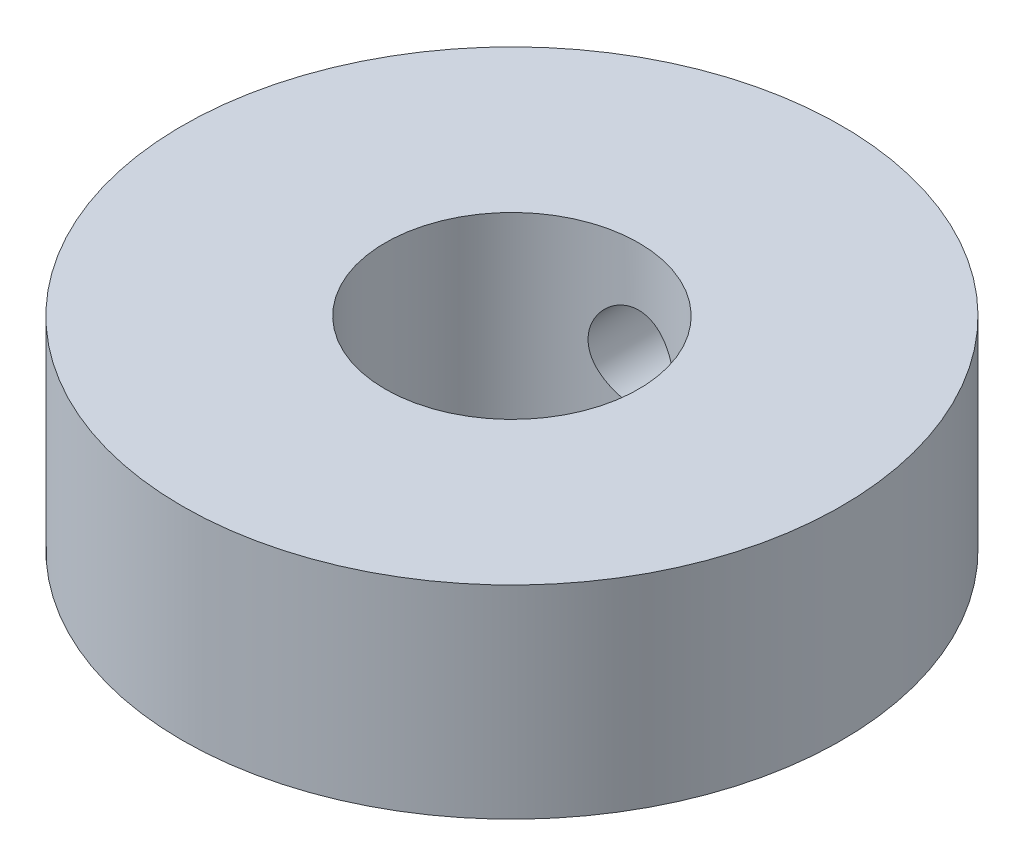
SolidWorks part; units mm, degrees
material "Plain Carbon Steel"
ref_plane "Front Plane" through (0, 0, 0) normal (0, 0, 1) x (1, 0, 0)
ref_plane "Top Plane" through (0, 0, 0) normal (0, 1, 0) x (1, 0, 0)
ref_plane "Right Plane" through (0, 0, 0) normal (1, 0, 0) x (0, 0, -1)
sketch "Ring Profile Ø13 x Ø5" plane through (0, 0, 0) normal (0, 1, 0) x (1, 0, 0)
  circle A0 centre (0, 0) radius 6.5
  circle A1 centre (0, 0) radius 2.5
  dimension "D1" = 13
  dimension "D2" = 5
extrude "Cover Ring" add sketch "Ring Profile Ø13 x Ø5" along normal blind 4
sketch "Radial Hole Profile Ø2" plane through (0, 0, 0) normal (0, 0, 1) x (1, 0, 0)
  circle A0 centre (0, 2) radius 0.85
  dimension "D1" = 2
  dimension "1.7" = 1.7
extrude "Radial Hole Ø2" cut sketch "Radial Hole Profile Ø2" against normal blind 7
